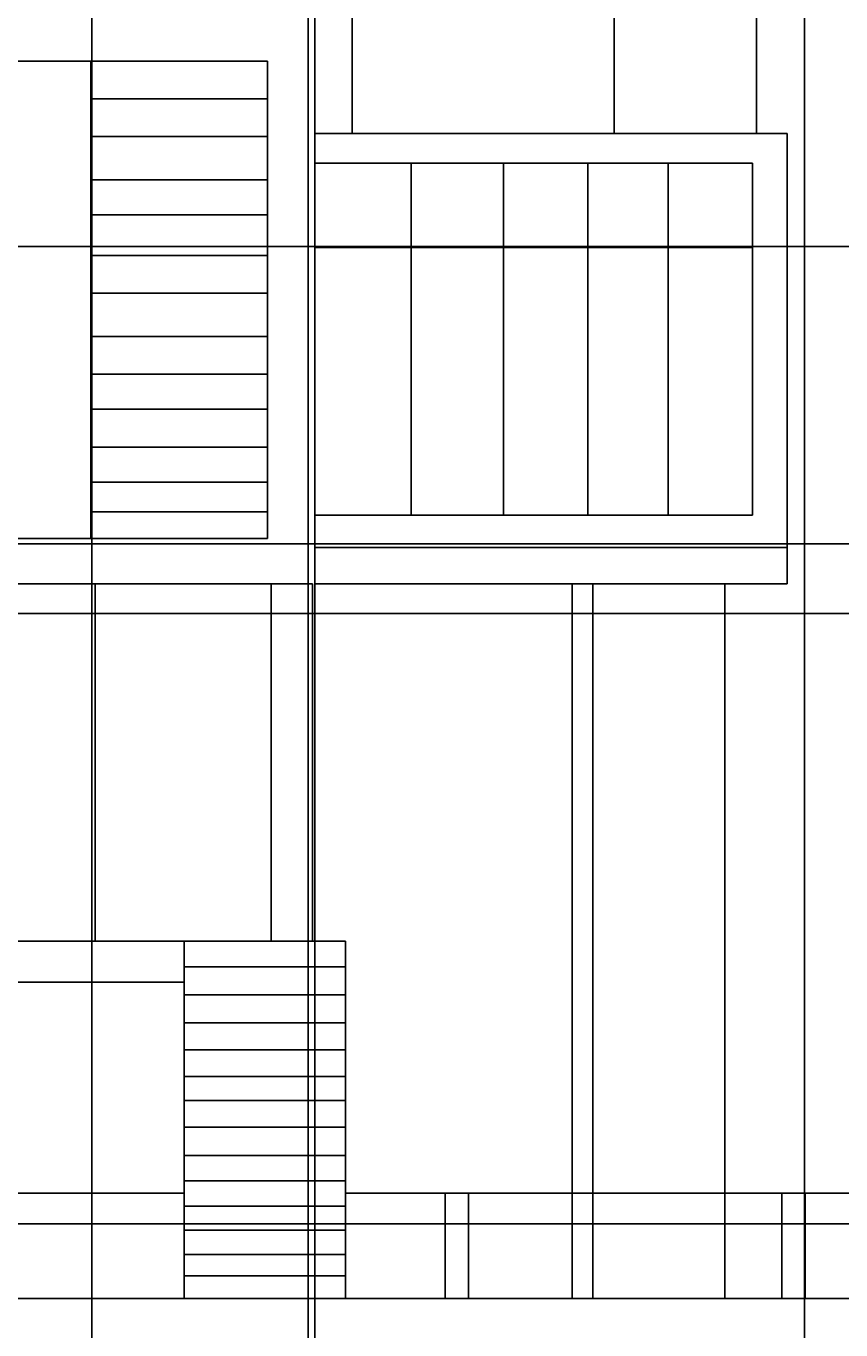
# Model space of a CAD drawing. Units: inches. Extents: x -117 to 121, y -77 to 40.
# Tile 26 of 45: x 50 to 72, y -43 to -8. Entities that reach past the tile are written whole.
import ezdxf

# ---------------------------------------------------------------- set-up
doc = ezdxf.new("R2010")
doc.units = ezdxf.units.IN
doc.header["$MEASUREMENT"] = 0
doc.layers.add('A-ANNO-DIMS', color=2, linetype='Continuous', lineweight=18)
doc.layers.add('A-ELEV', color=7, linetype='Continuous', lineweight=25)
doc.styles.get("Standard").update_dxf_attribs({"font": 'arial.ttf'})
doc.dimstyles.get("Standard").update_dxf_attribs({"dimtxt": 0.18, "dimasz": 0.18, "dimexe": 0.18, "dimexo": 0.0625, "dimgap": 0.09, "dimtad": 0, "dimtih": 1, "dimtoh": 1, "dimdec": 4, "dimzin": 0, "dimdsep": 46, "dimtxsty": 'Standard', "dimcen": 0.09, "dimadec": 0, "dimazin": 0, "dimtfac": 1, "dimtdec": 4, "dimtofl": 0, "dimtmove": 0, "dimatfit": 3, "dimfxl": 1, "dimtolj": 1, "dimtzin": 0, "dimarcsym": 0})

# ---------------------------------------------------------------- blocks, each defined once
blk = doc.blocks.new('*D33')
at = {"layer": 'A-ANNO-DIMS', "color": 0, "lineweight": -2, "transparency": 16777216}
for p, q in [((57.433, -43.571), (57.433, 38.61)), ((70.621, -43.571), (70.621, 38.61)), ((57.613, 38.43), (63.572, 38.43)), ((70.441, 38.43), (64.482, 38.43))]:
    blk.add_line(p, q, dxfattribs=at)
at = {"layer": 'A-ANNO-DIMS', "color": 0, "transparency": 16777216}
for points in [[(57.613, 38.46), (57.613, 38.4), (57.433, 38.43)], [(70.441, 38.46), (70.441, 38.4), (70.621, 38.43)]]:
    blk.add_solid(points, dxfattribs=at)
at = {"layer": 'Defpoints', "color": 0, "transparency": 16777216}
for p in [(70.621, 38.43), (57.433, -43.633), (70.621, -43.633)]:
    blk.add_point(p, dxfattribs=at)
at = {"layer": 'A-ANNO-DIMS', "color": 0, "transparency": 16777216, "insert": (64.027, 38.43), "char_height": 0.18, "attachment_point": 5}
blk.add_mtext('\\A1;13.189', dxfattribs=at)
blk = doc.blocks.new('*D49')
at = {"layer": 'A-ANNO-DIMS', "color": 0, "lineweight": -2, "transparency": 16777216}
for p, q in [((-45.422, -23.501), (120.84, -23.501)), ((120.66, -23.681), (120.66, -31.426)), ((120.66, -39.536), (120.66, -31.79)), ((-45.471, -39.716), (120.84, -39.716))]:
    blk.add_line(p, q, dxfattribs=at)
at = {"layer": 'A-ANNO-DIMS', "color": 0, "transparency": 16777216}
for points in [[(120.63, -23.681), (120.69, -23.681), (120.66, -23.501)], [(120.63, -39.536), (120.69, -39.536), (120.66, -39.716)]]:
    blk.add_solid(points, dxfattribs=at)
at = {"layer": 'Defpoints', "color": 0, "transparency": 16777216}
for p in [(-45.485, -23.501), (120.66, -23.501), (-45.533, -39.716)]:
    blk.add_point(p, dxfattribs=at)
at = {"layer": 'A-ANNO-DIMS', "color": 0, "transparency": 16777216, "insert": (120.66, -31.608), "char_height": 0.18, "attachment_point": 5}
blk.add_mtext('\\A1;16.215', dxfattribs=at)
blk = doc.blocks.new('*D50')
at = {"layer": 'A-ANNO-DIMS', "color": 0, "lineweight": -2, "transparency": 16777216}
for p, q in [((-47.458, -13.74), (120.84, -13.74)), ((120.66, -13.92), (120.66, -17.512)), ((120.66, -21.468), (120.66, -17.876)), ((-47.458, -21.648), (120.84, -21.648))]:
    blk.add_line(p, q, dxfattribs=at)
at = {"layer": 'A-ANNO-DIMS', "color": 0, "transparency": 16777216}
for points in [[(120.63, -13.92), (120.69, -13.92), (120.66, -13.74)], [(120.63, -21.468), (120.69, -21.468), (120.66, -21.648)]]:
    blk.add_solid(points, dxfattribs=at)
at = {"layer": 'Defpoints', "color": 0, "transparency": 16777216}
for p in [(-47.521, -13.74), (120.66, -13.74), (-47.521, -21.648)]:
    blk.add_point(p, dxfattribs=at)
at = {"layer": 'A-ANNO-DIMS', "color": 0, "transparency": 16777216, "insert": (120.66, -17.694), "char_height": 0.18, "attachment_point": 5}
blk.add_mtext('\\A1;7.908', dxfattribs=at)
blk = doc.blocks.new('*D53')
at = {"layer": 'A-ANNO-DIMS', "color": 0, "lineweight": -2, "transparency": 16777216}
for p, q in [((27.974, 10.841), (27.974, -77.193)), ((51.69, 10.9), (51.69, -77.193)), ((28.154, -77.013), (39.367, -77.013)), ((51.51, -77.013), (40.297, -77.013))]:
    blk.add_line(p, q, dxfattribs=at)
at = {"layer": 'A-ANNO-DIMS', "color": 0, "transparency": 16777216}
for points in [[(28.154, -76.983), (28.154, -77.043), (27.974, -77.013)], [(51.51, -76.983), (51.51, -77.043), (51.69, -77.013)]]:
    blk.add_solid(points, dxfattribs=at)
at = {"layer": 'Defpoints', "color": 0, "transparency": 16777216}
for p in [(27.974, 10.903), (51.69, 10.962), (51.69, -77.013)]:
    blk.add_point(p, dxfattribs=at)
at = {"layer": 'A-ANNO-DIMS', "color": 0, "transparency": 16777216, "insert": (39.832, -77.013), "char_height": 0.18, "attachment_point": 5}
blk.add_mtext('\\A1;23.716', dxfattribs=at)
blk = doc.blocks.new('*D58')
at = {"layer": 'A-ANNO-DIMS', "color": 0, "lineweight": -2, "transparency": 16777216}
for p, q in [((57.61, -7.947), (57.61, -77.193)), ((24.248, -8.105), (24.248, -77.193)), ((24.428, -77.013), (40.467, -77.013)), ((57.43, -77.013), (41.392, -77.013))]:
    blk.add_line(p, q, dxfattribs=at)
at = {"layer": 'A-ANNO-DIMS', "color": 0, "transparency": 16777216}
for points in [[(24.428, -76.983), (24.428, -77.043), (24.248, -77.013)], [(57.43, -76.983), (57.43, -77.043), (57.61, -77.013)]]:
    blk.add_solid(points, dxfattribs=at)
at = {"layer": 'Defpoints', "color": 0, "transparency": 16777216}
for p in [(57.61, -7.885), (24.248, -8.042), (57.61, -77.013)]:
    blk.add_point(p, dxfattribs=at)
at = {"layer": 'A-ANNO-DIMS', "color": 0, "transparency": 16777216, "insert": (40.929, -77.013), "char_height": 0.18, "attachment_point": 5}
blk.add_mtext('\\A1;33.362', dxfattribs=at)

msp = doc.modelspace()

# ---------------------------------------------------------------- linework, layer by layer
at = {"layer": 'A-ELEV'}
for p, q in [((57.6104, -2.6527), (57.6104, -10.7374)), ((65.562, -2.6527), (65.562, -10.7374)), ((69.3498, -2.6527), (69.3498, -10.7374)), ((58.6093, -6.5943), (58.6093, -10.7374)), ((56.354, -8.8134), (29.012, -8.8134)), ((51.666, -8.8134), (51.666, -21.5025)), ((56.354, -8.8134), (56.354, -21.5025)), ((56.354, -9.8179), (51.666, -9.8179)), ((58.6093, -10.7374), (57.6104, -10.7374)), ((57.6104, -10.7374), (57.6104, -21.7454)), ((58.6093, -10.7374), (70.1634, -10.7374)), ((70.1634, -10.7374), (70.1634, -21.7454)), ((56.354, -10.8224), (51.666, -10.8224)), ((57.6104, -11.531), (69.2364, -11.531)), ((60.1707, -11.531), (60.1707, -20.8857)), ((62.6237, -11.531), (62.6237, -20.8857)), ((64.8635, -11.531), (64.8635, -20.8857)), ((66.9966, -11.531), (66.9966, -20.8857)), ((69.2364, -11.531), (69.2364, -20.8857)), ((56.354, -11.9705), (51.666, -11.9705)), ((56.354, -12.9032), (51.666, -12.9032)), ((57.6104, -13.7681), (69.2364, -13.7681)), ((56.354, -13.9795), (51.666, -13.9795)), ((56.354, -14.984), (51.666, -14.984)), ((56.354, -16.1321), (51.666, -16.1321)), ((56.354, -17.1366), (51.666, -17.1366)), ((56.354, -18.0694), (51.666, -18.0694)), ((56.354, -19.0739), (51.666, -19.0739)), ((56.354, -20.0066), (51.666, -20.0066)), ((56.354, -20.7986), (51.666, -20.7986)), ((69.2364, -20.8857), (57.6104, -20.8857)), ((56.354, -21.5025), (29.012, -21.5025)), ((57.6104, -21.7454), (58.6093, -21.7454)), ((57.6104, -21.7454), (57.6104, -22.7074)), ((70.1634, -21.7454), (58.6093, -21.7454)), ((70.1634, -21.7454), (70.1634, -22.7074)), ((56.4528, -22.7074), (29.012, -22.7074)), ((51.7765, -22.7074), (51.7765, -32.2104)), ((56.4528, -22.7074), (56.4528, -32.2104)), ((57.5488, -22.7074), (56.4528, -22.7074)), ((57.5488, -22.7074), (57.5488, -32.2104)), ((57.6104, -22.7074), (58.6093, -22.7074)), ((70.1634, -22.7074), (58.6093, -22.7074)), ((64.4531, -22.7074), (64.4531, -41.7053)), ((65.0011, -22.7074), (65.0011, -41.7053)), ((68.508, -22.7074), (68.508, -41.7053)), ((54.143, -32.2104), (38.4517, -32.2104)), ((54.143, -32.2104), (54.143, -41.7053)), ((54.143, -32.2104), (58.4308, -32.2104)), ((58.4308, -32.2104), (58.4308, -41.7053)), ((54.143, -32.886), (58.4308, -32.886)), ((38.4517, -33.2923), (54.143, -33.2923)), ((54.143, -33.6327), (58.4308, -33.6327)), ((54.143, -34.3793), (58.4308, -34.3793)), ((54.143, -35.0905), (58.4308, -35.0905)), ((54.143, -35.8016), (58.4308, -35.8016)), ((54.143, -36.4416), (58.4308, -36.4416)), ((54.143, -37.1528), (58.4308, -37.1528)), ((54.143, -37.8994), (58.4308, -37.8994)), ((54.143, -38.575), (58.4308, -38.575)), ((21.9795, -38.9022), (54.143, -38.9022)), ((58.4308, -38.9022), (72.4671, -38.9022)), ((61.0794, -41.7053), (61.0794, -38.9022)), ((61.6931, -41.7053), (61.6931, -38.9022)), ((70.0215, -41.7053), (70.0215, -38.9022)), ((70.6352, -41.7053), (70.6352, -38.9022)), ((54.143, -39.2506), (58.4308, -39.2506)), ((54.143, -39.8906), (58.4308, -39.8906)), ((54.143, -40.5306), (58.4308, -40.5306)), ((54.143, -41.0995), (58.4308, -41.0995)), ((68.508, -41.7053), (37.6294, -41.7053)), ((72.4671, -41.7053), (68.508, -41.7053))]:
    msp.add_line(p, q, dxfattribs=at)

# ---------------------------------------------------------------- dimensions: what is measured, and where the dimension line sits
at = {"layer": 'A-ANNO-DIMS'}
for base, p1, p2, picture, middle in [((70.6214, 38.4297), (57.4328, -43.6334), (70.6214, -43.6334), '*D33', (64.0271, 38.4297)), ((51.6901, -77.0135), (27.9744, 10.9032), (51.6901, 10.9623), '*D53', (39.8322, -77.0135)), ((57.6104, -77.0135), (24.2481, -8.0421), (57.6104, -7.8846), '*D58', (40.9293, -77.0135))]:
    dim = msp.add_linear_dim(base=base, p1=p1, p2=p2, dimstyle='Standard', override={"dimdec": 3, "dimlfac": 1, "dimrnd": 0, "dimzin": 0, "dimdsep": 46, "dimlunit": 2}, dxfattribs=at)
    dim.commit()
    dim.dimension.update_dxf_attribs({"geometry": picture, "text_midpoint": middle})
for base, p1, p2, picture, middle in [((120.6602, -13.74), (-47.5206, -21.6476), (-47.5206, -13.74), '*D50', (120.6602, -17.6938)), ((120.6602, -23.5007), (-45.5331, -39.716), (-45.4848, -23.5007), '*D49', (120.6602, -31.6083))]:
    dim = msp.add_linear_dim(base=base, p1=p1, p2=p2, angle=90, dimstyle='Standard', override={"dimdec": 3, "dimlfac": 1, "dimrnd": 0, "dimzin": 0, "dimdsep": 46, "dimlunit": 2}, dxfattribs=at)
    dim.commit()
    dim.dimension.update_dxf_attribs({"geometry": picture, "text_midpoint": middle})

doc.saveas('drawing.dxf')
